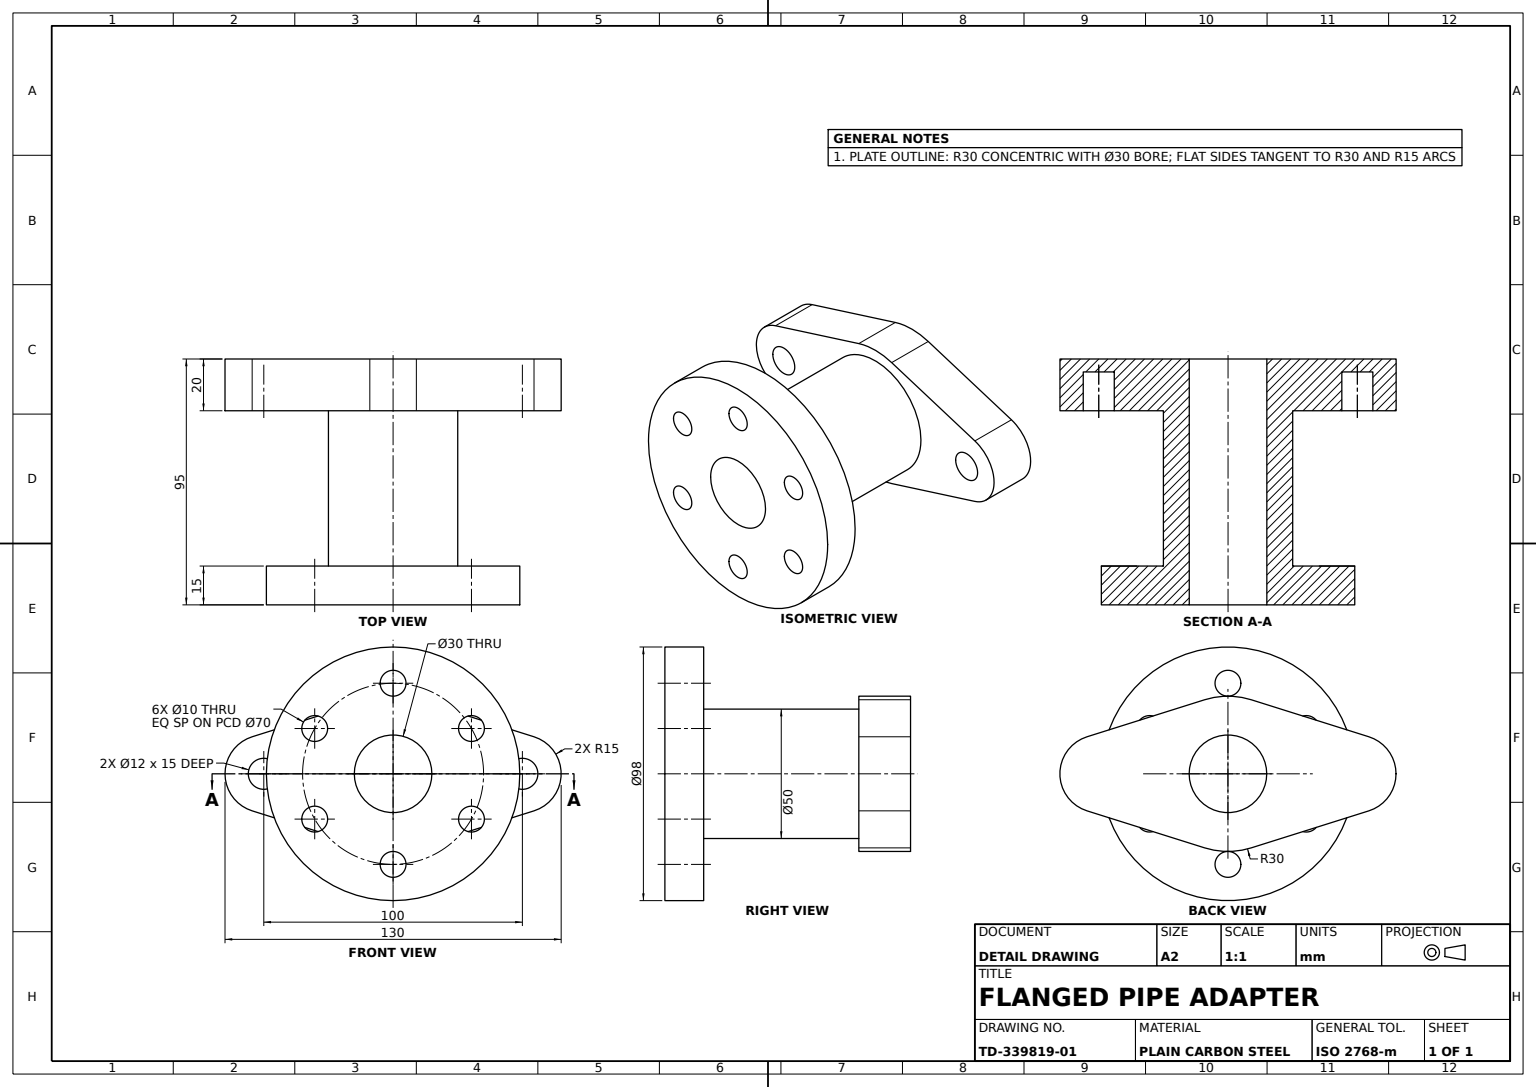
SolidWorks part; units mm, degrees
material "Plain Carbon Steel"
ref_plane "Front Plane" through (0, 0, 0) normal (0, 0, 1) x (1, 0, 0)
ref_plane "Top Plane" through (0, 0, 0) normal (0, 1, 0) x (1, 0, 0)
ref_plane "Right Plane" through (0, 0, 0) normal (1, 0, 0) x (0, 0, -1)
sketch "Mounting Plate Sketch" plane through (0, 0, 0) normal (0, 0, 1) x (1, 0, 0)
  line L0 (0, 0) -> (50, 0) construction
  line L1 (50, 0) -> (100, 0) construction
  line L2 (-4.5, 14.3091) -> (41, 28.6182)
  line L3 (-4.5, -14.3091) -> (41, -28.6182)
  line L4 (59, 28.6182) -> (104.5, 14.3091)
  line L5 (59, -28.6182) -> (104.5, -14.3091)
  arc A0 (-4.5, 14.3091) -> (-4.5, -14.3091) centre (0, 0) ccw
  arc A1 (104.5, -14.3091) -> (104.5, 14.3091) centre (100, 0) ccw
  arc A2 (41, -28.6182) -> (59, -28.6182) centre (50, 0) ccw
  arc A3 (59, 28.6182) -> (41, 28.6182) centre (50, 0) ccw
  dimension "D1" = 30
  dimension "D2" = 30
  dimension "D3" = 50
  dimension "D5" = 60
  dimension "D4" = 100
extrude "Mounting Plate" add sketch "Mounting Plate Sketch" along normal blind 20
sketch "Hub Sketch" plane through (0, 0, 20) normal (0, 0, 1) x (1, 0, 0)
  circle A0 centre (50, 0) radius 25
  dimension "D1" = 50
extrude "Hub Ø50" add sketch "Hub Sketch" along normal blind 60
sketch "Flange Sketch" plane through (0, 0, 80) normal (0, 0, 1) x (1, 0, 0)
  circle A0 centre (50, 0) radius 49
  dimension "D1" = 98
extrude "Flange Ø98" add sketch "Flange Sketch" along normal blind 15
sketch "Flange Bolt Hole Sketch" plane through (0, 0, 95) normal (0, 0, 1) x (1, 0, 0)
  line L0 (50, 0) -> (50, 35) construction
  circle A0 centre (50, 0) radius 35 construction
  circle A1 centre (50, 35) radius 5
  dimension "D1" = 10
  dimension "D2" = 70
extrude "Flange Bolt Hole Ø10" cut sketch "Flange Bolt Hole Sketch" against normal blind 15
sketch "Bore Sketch" plane through (0, 0, 95) normal (0, 0, 1) x (1, 0, 0)
  circle A0 centre (50, 0) radius 15
  dimension "D1" = 30
extrude "Bore Cut" cut sketch "Bore Sketch" against normal through all
pattern_circular "Flange Bolt Hole Pattern 6x" count 6 over 360 about axis through (50, 0, 0) along (0, 0, 1) of "Flange Bolt Hole Ø10"
sketch "Plate Holes Sketch" plane through (0, 0, 20) normal (0, 0, 1) x (1, 0, 0)
  circle A0 centre (0, 0) radius 6
  circle A1 centre (100, 0) radius 6
  dimension "D1" = 12
  dimension "D2" = 12
extrude "Plate Holes 2xØ12" cut sketch "Plate Holes Sketch" against normal blind 15
